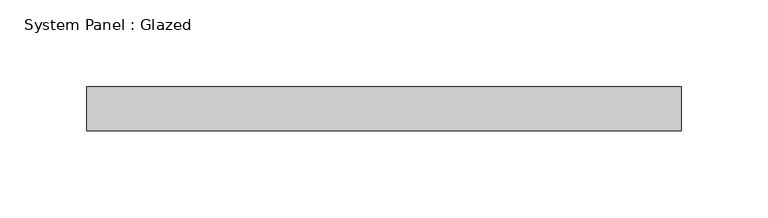
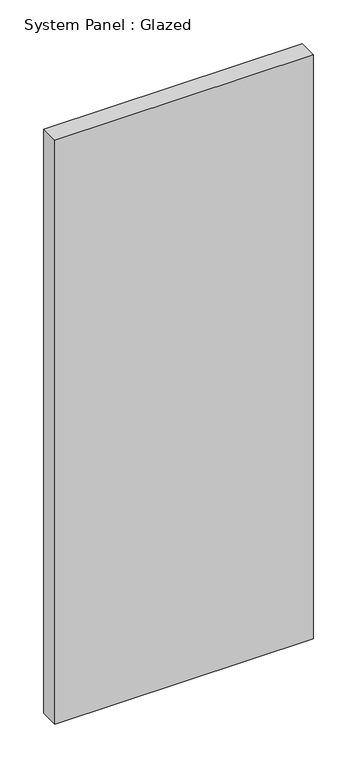
"""IFC4 building model written with IfcOpenShell, lengths in millimetres: plate geometry, System Panel : Glazed."""

from ifc_helpers import new_model, si_unit, origin, origin_with_axes, place, context, project, spatial, polyline, outline, extrude, source, transform, mapped, element, save


def system_panel_glazed_6255ac7b(model_context):
    return source(origin(), model_context, "Body", "SweptSolid", [
        extrude(outline(polyline([(171.45, 19.05), (-171.45, 19.05), (-171.45, 44.45), (171.45, 44.45), (171.45, 19.05)])), origin_with_axes(), (0.0, 0.0, 1.0), 818.8480012),
    ])


if __name__ == "__main__":
    model = new_model("IFC4")
    model_context = context("Model", 3, world=origin())
    ifc_project = project(units=[si_unit("LENGTHUNIT", "METRE", prefix="MILLI")], contexts=[model_context])
    site = spatial("IfcSite", under=ifc_project)
    building = spatial("IfcBuilding", under=site)
    placement = place(None, origin())
    system_panel_glazed_shape = system_panel_glazed_6255ac7b(model_context)
    element("IfcPlate", 1, ObjectType="System Panel : Glazed", at=placement, inside=building, context=model_context, shape_type="MappedRepresentation", body=[
        mapped(system_panel_glazed_shape, transform((0.0, 0.0, 0.0), x_axis=(1.0, 0.0, 0.0), y_axis=(0.0, 1.0, 0.0), z_axis=(0.0, 0.0, 1.0))),
    ])
    save(model, "model.ifc")

# Revit data of these elements
# Type "System Panel : Glazed"
#   Construction Type Id = "GSP4R"
#   Analytic Construction = "1/8 in Pilkington single glazing"
#   Visual Light Transmittance = 0.9
#   Solar Heat Gain Coefficient = 0.86
#   Heat Transfer Coefficient (U) = 1.18115 BTU/(h·ft²·°F)
# Element 1 (IfcPlate, "System Panel : Glazed")
#   Materials on its faces: "Glass"
# Materials
#   "Glass": class "Glass", colour RGB 0 128 192, transparency 0.75, Description = "Soda Lime Glass", Cost = 0
